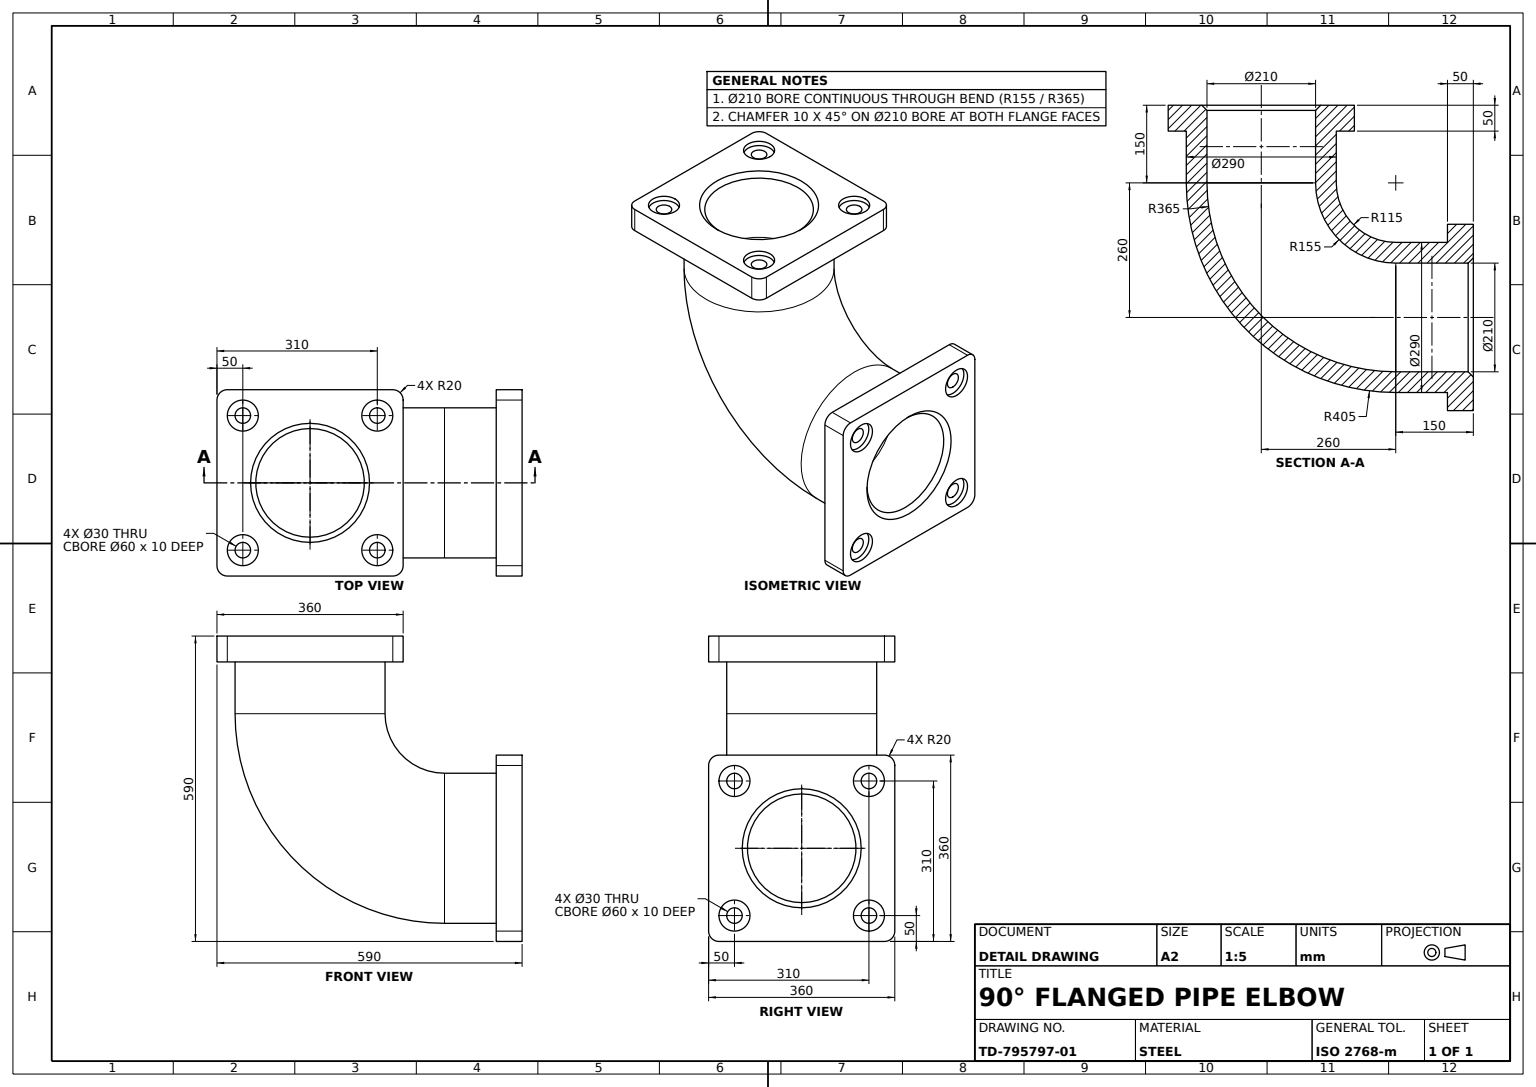
SolidWorks part; units mm, degrees
material "Plain Carbon Steel"
ref_plane "Front Plane" through (0, 0, 0) normal (0, 0, 1) x (1, 0, 0)
ref_plane "Top Plane" through (0, 0, 0) normal (0, 1, 0) x (1, 0, 0)
ref_plane "Right Plane" through (0, 0, 0) normal (1, 0, 0) x (0, 0, -1)
sketch "Elbow Path Sketch" plane through (0, 0, 0) normal (0, 0, 1) x (1, 0, 0)
  line L0 (0, 0) -> (-150, 0)
  line L1 (-410, 260) -> (-410, 410)
  arc A0 (-150, 0) -> (-410, 260) centre (-150, 260) cw
  dimension "D1" = 260
  dimension "D2" = 150
sketch "Pipe Profile Sketch Ø290" plane through (0, 0, 0) normal (1, 0, 0) x (0, 0, -1)
  circle A0 centre (0, 0) radius 145
  dimension "D1" = 290
sweep "Elbow Pipe Sweep Wall 40" add profiles "Pipe Profile Sketch Ø290" path "Elbow Path Sketch" parameters "D1"=40
sketch "Flange A Sketch 360x360" plane through (0, 0, 0) normal (1, 0, 0) x (0, 0, -1)
  line L1 (-180, 180) -> (180, 180)
  line L2 (-180, 180) -> (-180, -180)
  line L3 (-180, -180) -> (180, -180)
  line L4 (180, 180) -> (180, -180)
  line L5 (-180, 180) -> (180, -180) construction
  line L6 (-180, -180) -> (180, 180) construction
  point P0 (0, 0)
  circle M6 centre (0, 0) radius 145
  dimension "D1" = 360
  dimension "D2" = 360
extrude "Flange A 360x360x50" add sketch "Flange A Sketch 360x360" against normal blind 50 contours L4 L1 L2 L3 M6
fillet "Flange A Corner Fillets R20" radius 20 4 edges at (-25, 180, -180) (-25, -180, 180) (-25, -180, -180) (-25, 180, 180)
sketch "Flange B Sketch 360x360" plane through (0, 410, 0) normal (0, 1, 0) x (1, 0, 0)
  line L1 (-590, 180) -> (-230, 180)
  line L2 (-590, 180) -> (-590, -180)
  line L3 (-590, -180) -> (-230, -180)
  line L4 (-230, 180) -> (-230, -180)
  line L5 (-590, 180) -> (-230, -180) construction
  line L6 (-590, -180) -> (-230, 180) construction
  point P0 (-410, 0)
  circle M6 centre (-410, 0) radius 145
  dimension "D1" = 360
  dimension "D2" = 360
extrude "Flange B 360x360x50" add sketch "Flange B Sketch 360x360" against normal blind 50 contours L4 L1 L2 L3 M6
fillet "Flange B Corner Fillets R20" radius 20 4 edges at (-230, 385, -180) (-590, 385, -180) (-230, 385, 180) (-590, 385, 180)
sketch "Flange A Counterbore Sketch Ø60" plane through (0, 0, 0) normal (1, 0, 0) x (0, 0, -1)
  line L2 (-130, 130) -> (130, 130) construction
  line L3 (-130, 130) -> (-130, -130) construction
  line L4 (-130, -130) -> (130, -130) construction
  line L5 (130, 130) -> (130, -130) construction
  line L6 (-130, 130) -> (130, -130) construction
  line L7 (-130, -130) -> (130, 130) construction
  circle A0 centre (-130, 130) radius 30
  point P2 (0, 0)
  dimension "D1" = 60
  dimension "D2" = 260
  dimension "D3" = 260
  dimension "D4" = 260
  dimension "D5" = 260
extrude "Flange A Counterbore Ø60x10" cut sketch "Flange A Counterbore Sketch Ø60" against normal blind 10
sketch "Flange A Bolt Hole Sketch Ø30" plane through (-10, 0, 0) normal (1, 0, 0) x (0, 0, -1)
  circle A0 centre (-130, 130) radius 15
  dimension "D1" = 30
extrude "Flange A Bolt Hole Ø30" cut sketch "Flange A Bolt Hole Sketch Ø30" against normal up to next
pattern_circular "Flange A Bolt Hole Pattern 4x" count 4 over 360 about axis through (0, 0, 0) along (1, 0, 0) of "Flange A Bolt Hole Ø30", "Flange A Counterbore Ø60x10"
sketch "Flange B Counterbore Sketch Ø60" plane through (0, 410, 0) normal (0, 1, 0) x (1, 0, 0)
  line L1 (-540, 130) -> (-280, 130) construction
  line L2 (-540, 130) -> (-540, -130) construction
  line L3 (-540, -130) -> (-280, -130) construction
  line L4 (-280, 130) -> (-280, -130) construction
  line L5 (-540, 130) -> (-280, -130) construction
  line L6 (-540, -130) -> (-280, 130) construction
  circle A0 centre (-540, 130) radius 30
  point P0 (-410, 0)
  dimension "D3" = 60
  dimension "D1" = 260
  dimension "D2" = 260
extrude "Flange B Counterbore Ø60x10" cut sketch "Flange B Counterbore Sketch Ø60" against normal blind 10
sketch "Flange B Bolt Hole Sketch Ø30" plane through (0, 400, 0) normal (0, 1, 0) x (1, 0, 0)
  circle A0 centre (-540, 130) radius 15
  dimension "D1" = 30
extrude "Flange B Bolt Hole Ø30" cut sketch "Flange B Bolt Hole Sketch Ø30" against normal up to next
pattern_circular "Flange B Bolt Hole Pattern 4x" count 4 over 360 about axis through (-410, 0, 0) along (0, 1, 0) of "Flange B Bolt Hole Ø30", "Flange B Counterbore Ø60x10"
chamfer "Pipe Edge Chamfer 10x45deg" distance 10 angle 45 2 edges at (0, 0, -105) (-305, 410, 0)
